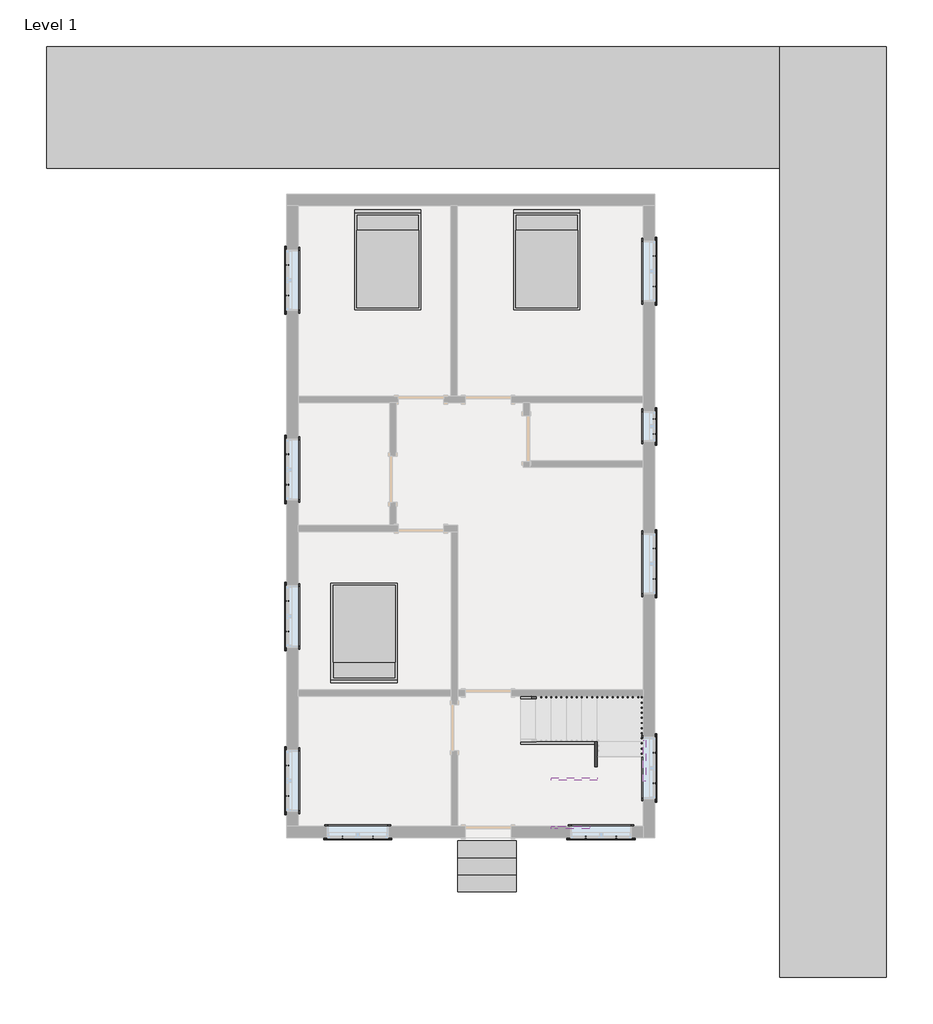
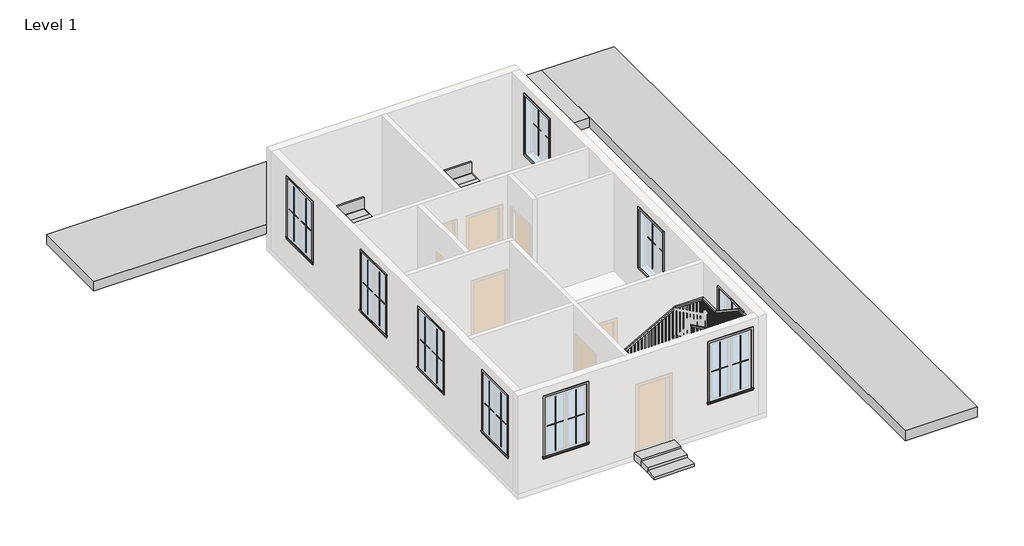
# One storey, part 2 of 2: 43 proxies, 6 members, 3 furniture elements, 1 railing.
"""IFC4 building model written with IfcOpenShell, lengths in millimetres."""

from ifc_helpers import new_model, si_unit, frame, origin, place, context, project, spatial, polyline, outline, extrude, faceted_brep, transform, mapped, element, save
from components import generic_models_1_generic_models_1_13bb2270, generic_models_2_generic_models_2_8d9d6b08, generic_models_3_generic_models_3_c7f04afc, muntin_pattern_2x2_muntin_pattern_2x2_2b4d9f72, muntin_pattern_2x2_muntin_pattern_2x2_ef995ed3, muntin_pattern_2x2_muntin_pattern_2x2_53152e2c, muntin_pattern_2x2_muntin_pattern_2x2_e8f3e573, trim_window_exterior_flat_with_sill_b7e4d11c, trim_window_exterior_flat_with_sill_a665a915, trim_window_interior_flat_picture_frame_936b8d2a, trim_window_interior_flat_picture_frame_d485c387, bed_17739_bed_17739_15c61121

model = new_model("IFC4")

# Units and contexts
model_context = context("Model", 3, world=origin())
ifc_project = project(units=[si_unit("LENGTHUNIT", "METRE", prefix="MILLI")], contexts=[model_context])

# Site, building, storey
site = spatial("IfcSite", under=ifc_project)
building = spatial("IfcBuilding", under=site)
storey = spatial("IfcBuildingStorey", under=building, Name="Level 1", Elevation=0.0)

# Proxies
placement = place(None, origin())
generic_models_1_generic_models_1_shape = generic_models_1_generic_models_1_13bb2270(model_context)
element("IfcBuildingElementProxy", 1, Name="Generic Models 1 : Generic Models 1", ObjectType="Generic Models 1 : Generic Models 1", at=placement, inside=storey, context=model_context, shape_type="MappedRepresentation", body=[
    mapped(generic_models_1_generic_models_1_shape, transform((0.0, 0.0, 0.0), x_axis=(1.0, 0.0, 0.0), y_axis=(0.0, 1.0, 0.0), z_axis=(0.0, 0.0, 1.0))),
])
generic_models_2_generic_models_2_shape = generic_models_2_generic_models_2_8d9d6b08(model_context)
element("IfcBuildingElementProxy", 2, Name="Generic Models 2 : Generic Models 2", ObjectType="Generic Models 2 : Generic Models 2", at=placement, inside=storey, context=model_context, shape_type="MappedRepresentation", body=[
    mapped(generic_models_2_generic_models_2_shape, transform((0.0, 0.0, 0.0), x_axis=(1.0, 0.0, 0.0), y_axis=(0.0, 1.0, 0.0), z_axis=(0.0, 0.0, 1.0))),
])
generic_models_3_generic_models_3_shape = generic_models_3_generic_models_3_c7f04afc(model_context)
element("IfcBuildingElementProxy", 3, Name="Generic Models 3 : Generic Models 3", ObjectType="Generic Models 3 : Generic Models 3", at=placement, inside=storey, context=model_context, shape_type="MappedRepresentation", body=[
    mapped(generic_models_3_generic_models_3_shape, transform((0.0, 0.0, 0.0), x_axis=(1.0, 0.0, 0.0), y_axis=(0.0, 1.0, 0.0), z_axis=(0.0, 0.0, 1.0))),
])
muntin_pattern_2x2_muntin_pattern_2x2_shape = muntin_pattern_2x2_muntin_pattern_2x2_2b4d9f72(model_context)
element("IfcBuildingElementProxy", 4, Name="Muntin Pattern_2x2 : Muntin Pattern_2x2", ObjectType="Muntin Pattern_2x2 : Muntin Pattern_2x2", at=placement, inside=storey, context=model_context, shape_type="MappedRepresentation", body=[
    mapped(muntin_pattern_2x2_muntin_pattern_2x2_shape, transform((1025.525, 12434.8875, 984.25), x_axis=(0.0, 1.0, 0.0), y_axis=(-1.0, 0.0, 0.0), z_axis=(0.0, 0.0, 1.0))),
])
element("IfcBuildingElementProxy", 5, Name="Muntin Pattern_2x2 : Muntin Pattern_2x2", ObjectType="Muntin Pattern_2x2 : Muntin Pattern_2x2", at=placement, inside=storey, context=model_context, shape_type="MappedRepresentation", body=[
    mapped(muntin_pattern_2x2_muntin_pattern_2x2_shape, transform((8321.675, 13219.1125, 984.25), x_axis=(0.0, -1.0, 0.0), y_axis=(1.0, 0.0, 0.0), z_axis=(0.0, 0.0, 1.0))),
])
element("IfcBuildingElementProxy", 6, Name="Muntin Pattern_2x2 : Muntin Pattern_2x2", ObjectType="Muntin Pattern_2x2 : Muntin Pattern_2x2", at=placement, inside=storey, context=model_context, shape_type="MappedRepresentation", body=[
    mapped(muntin_pattern_2x2_muntin_pattern_2x2_shape, transform((8321.675, 3338.5125, 984.25), x_axis=(0.0, -1.0, 0.0), y_axis=(1.0, 0.0, 0.0), z_axis=(0.0, 0.0, 1.0))),
])
element("IfcBuildingElementProxy", 7, Name="Muntin Pattern_2x2 : Muntin Pattern_2x2", ObjectType="Muntin Pattern_2x2 : Muntin Pattern_2x2", at=placement, inside=storey, context=model_context, shape_type="MappedRepresentation", body=[
    mapped(muntin_pattern_2x2_muntin_pattern_2x2_shape, transform((7567.6125, 1660.525, 984.25), x_axis=(-1.0, 0.0, 0.0), y_axis=(0.0, -1.0, 0.0), z_axis=(0.0, 0.0, 1.0))),
])
element("IfcBuildingElementProxy", 8, Name="Muntin Pattern_2x2 : Muntin Pattern_2x2", ObjectType="Muntin Pattern_2x2 : Muntin Pattern_2x2", at=placement, inside=storey, context=model_context, shape_type="MappedRepresentation", body=[
    mapped(muntin_pattern_2x2_muntin_pattern_2x2_shape, transform((2728.9125, 1660.525, 984.25), x_axis=(-1.0, 0.0, 0.0), y_axis=(0.0, -1.0, 0.0), z_axis=(0.0, 0.0, 1.0))),
])
element("IfcBuildingElementProxy", 9, Name="Muntin Pattern_2x2 : Muntin Pattern_2x2", ObjectType="Muntin Pattern_2x2 : Muntin Pattern_2x2", at=placement, inside=storey, context=model_context, shape_type="MappedRepresentation", body=[
    mapped(muntin_pattern_2x2_muntin_pattern_2x2_shape, transform((1025.525, 2478.0875, 984.25), x_axis=(0.0, 1.0, 0.0), y_axis=(-1.0, 0.0, 0.0), z_axis=(0.0, 0.0, 1.0))),
])
element("IfcBuildingElementProxy", 10, Name="Muntin Pattern_2x2 : Muntin Pattern_2x2", ObjectType="Muntin Pattern_2x2 : Muntin Pattern_2x2", at=placement, inside=storey, context=model_context, shape_type="MappedRepresentation", body=[
    mapped(muntin_pattern_2x2_muntin_pattern_2x2_shape, transform((1025.525, 5748.3375, 984.25), x_axis=(0.0, 1.0, 0.0), y_axis=(-1.0, 0.0, 0.0), z_axis=(0.0, 0.0, 1.0))),
])
element("IfcBuildingElementProxy", 11, Name="Muntin Pattern_2x2 : Muntin Pattern_2x2", ObjectType="Muntin Pattern_2x2 : Muntin Pattern_2x2", at=placement, inside=storey, context=model_context, shape_type="MappedRepresentation", body=[
    mapped(muntin_pattern_2x2_muntin_pattern_2x2_shape, transform((1025.525, 8669.3375, 984.25), x_axis=(0.0, 1.0, 0.0), y_axis=(-1.0, 0.0, 0.0), z_axis=(0.0, 0.0, 1.0))),
])
element("IfcBuildingElementProxy", 12, Name="Muntin Pattern_2x2 : Muntin Pattern_2x2", ObjectType="Muntin Pattern_2x2 : Muntin Pattern_2x2", at=placement, inside=storey, context=model_context, shape_type="MappedRepresentation", body=[
    mapped(muntin_pattern_2x2_muntin_pattern_2x2_shape, transform((8321.675, 7402.5125, 984.25), x_axis=(0.0, -1.0, 0.0), y_axis=(1.0, 0.0, 0.0), z_axis=(0.0, 0.0, 1.0))),
])
muntin_pattern_2x2_muntin_pattern_2x2_2_shape = muntin_pattern_2x2_muntin_pattern_2x2_ef995ed3(model_context)
element("IfcBuildingElementProxy", 13, Name="Muntin Pattern_2x2 : Muntin Pattern_2x2", ObjectType="Muntin Pattern_2x2 : Muntin Pattern_2x2", at=placement, inside=storey, context=model_context, shape_type="MappedRepresentation", body=[
    mapped(muntin_pattern_2x2_muntin_pattern_2x2_2_shape, transform((1025.525, 13041.3125, 984.25), x_axis=(0.0, -1.0, 0.0), y_axis=(1.0, 0.0, 0.0), z_axis=(0.0, 0.0, 1.0))),
])
element("IfcBuildingElementProxy", 14, Name="Muntin Pattern_2x2 : Muntin Pattern_2x2", ObjectType="Muntin Pattern_2x2 : Muntin Pattern_2x2", at=placement, inside=storey, context=model_context, shape_type="MappedRepresentation", body=[
    mapped(muntin_pattern_2x2_muntin_pattern_2x2_2_shape, transform((8321.675, 12612.6875, 984.25), x_axis=(0.0, 1.0, 0.0), y_axis=(-1.0, 0.0, 0.0), z_axis=(0.0, 0.0, 1.0))),
])
element("IfcBuildingElementProxy", 15, Name="Muntin Pattern_2x2 : Muntin Pattern_2x2", ObjectType="Muntin Pattern_2x2 : Muntin Pattern_2x2", at=placement, inside=storey, context=model_context, shape_type="MappedRepresentation", body=[
    mapped(muntin_pattern_2x2_muntin_pattern_2x2_2_shape, transform((8321.675, 2732.0875, 984.25), x_axis=(0.0, 1.0, 0.0), y_axis=(-1.0, 0.0, 0.0), z_axis=(0.0, 0.0, 1.0))),
])
element("IfcBuildingElementProxy", 16, Name="Muntin Pattern_2x2 : Muntin Pattern_2x2", ObjectType="Muntin Pattern_2x2 : Muntin Pattern_2x2", at=placement, inside=storey, context=model_context, shape_type="MappedRepresentation", body=[
    mapped(muntin_pattern_2x2_muntin_pattern_2x2_2_shape, transform((6961.1875, 1660.525, 984.25), x_axis=(1.0, 0.0, 0.0), y_axis=(0.0, 1.0, 0.0), z_axis=(0.0, 0.0, 1.0))),
])
element("IfcBuildingElementProxy", 17, Name="Muntin Pattern_2x2 : Muntin Pattern_2x2", ObjectType="Muntin Pattern_2x2 : Muntin Pattern_2x2", at=placement, inside=storey, context=model_context, shape_type="MappedRepresentation", body=[
    mapped(muntin_pattern_2x2_muntin_pattern_2x2_2_shape, transform((2122.4875, 1660.525, 984.25), x_axis=(1.0, 0.0, 0.0), y_axis=(0.0, 1.0, 0.0), z_axis=(0.0, 0.0, 1.0))),
])
element("IfcBuildingElementProxy", 18, Name="Muntin Pattern_2x2 : Muntin Pattern_2x2", ObjectType="Muntin Pattern_2x2 : Muntin Pattern_2x2", at=placement, inside=storey, context=model_context, shape_type="MappedRepresentation", body=[
    mapped(muntin_pattern_2x2_muntin_pattern_2x2_2_shape, transform((1025.525, 3084.5125, 984.25), x_axis=(0.0, -1.0, 0.0), y_axis=(1.0, 0.0, 0.0), z_axis=(0.0, 0.0, 1.0))),
])
element("IfcBuildingElementProxy", 19, Name="Muntin Pattern_2x2 : Muntin Pattern_2x2", ObjectType="Muntin Pattern_2x2 : Muntin Pattern_2x2", at=placement, inside=storey, context=model_context, shape_type="MappedRepresentation", body=[
    mapped(muntin_pattern_2x2_muntin_pattern_2x2_2_shape, transform((1025.525, 6354.7625, 984.25), x_axis=(0.0, -1.0, 0.0), y_axis=(1.0, 0.0, 0.0), z_axis=(0.0, 0.0, 1.0))),
])
element("IfcBuildingElementProxy", 20, Name="Muntin Pattern_2x2 : Muntin Pattern_2x2", ObjectType="Muntin Pattern_2x2 : Muntin Pattern_2x2", at=placement, inside=storey, context=model_context, shape_type="MappedRepresentation", body=[
    mapped(muntin_pattern_2x2_muntin_pattern_2x2_2_shape, transform((1025.525, 9275.7625, 984.25), x_axis=(0.0, -1.0, 0.0), y_axis=(1.0, 0.0, 0.0), z_axis=(0.0, 0.0, 1.0))),
])
element("IfcBuildingElementProxy", 21, Name="Muntin Pattern_2x2 : Muntin Pattern_2x2", ObjectType="Muntin Pattern_2x2 : Muntin Pattern_2x2", at=placement, inside=storey, context=model_context, shape_type="MappedRepresentation", body=[
    mapped(muntin_pattern_2x2_muntin_pattern_2x2_2_shape, transform((8321.675, 6796.0875, 984.25), x_axis=(0.0, 1.0, 0.0), y_axis=(-1.0, 0.0, 0.0), z_axis=(0.0, 0.0, 1.0))),
])
muntin_pattern_2x2_muntin_pattern_2x2_3_shape = muntin_pattern_2x2_muntin_pattern_2x2_53152e2c(model_context)
element("IfcBuildingElementProxy", 22, Name="Muntin Pattern_2x2 : Muntin Pattern_2x2", ObjectType="Muntin Pattern_2x2 : Muntin Pattern_2x2", at=placement, inside=storey, context=model_context, shape_type="MappedRepresentation", body=[
    mapped(muntin_pattern_2x2_muntin_pattern_2x2_3_shape, transform((8321.675, 9980.6125, 984.25), x_axis=(0.0, -1.0, 0.0), y_axis=(1.0, 0.0, 0.0), z_axis=(0.0, 0.0, 1.0))),
])
muntin_pattern_2x2_muntin_pattern_2x2_4_shape = muntin_pattern_2x2_muntin_pattern_2x2_e8f3e573(model_context)
element("IfcBuildingElementProxy", 23, Name="Muntin Pattern_2x2 : Muntin Pattern_2x2", ObjectType="Muntin Pattern_2x2 : Muntin Pattern_2x2", at=placement, inside=storey, context=model_context, shape_type="MappedRepresentation", body=[
    mapped(muntin_pattern_2x2_muntin_pattern_2x2_4_shape, transform((8321.675, 9678.9875, 984.25), x_axis=(0.0, 1.0, 0.0), y_axis=(-1.0, 0.0, 0.0), z_axis=(0.0, 0.0, 1.0))),
])
trim_window_exterior_flat_with_sill_shape = trim_window_exterior_flat_with_sill_b7e4d11c(model_context)
element("IfcBuildingElementProxy", 24, Name="Trim-Window-Exterior-Flat : with Sill", ObjectType="Trim-Window-Exterior-Flat : with Sill", at=placement, inside=storey, context=model_context, shape_type="MappedRepresentation", body=[
    mapped(trim_window_exterior_flat_with_sill_shape, transform((1016.0, 12738.1, 2743.2), x_axis=(0.0, -1.0, 0.0), y_axis=(0.0, 0.0, 1.0), z_axis=(-1.0, 0.0, 0.0))),
])
element("IfcBuildingElementProxy", 25, Name="Trim-Window-Exterior-Flat : with Sill", ObjectType="Trim-Window-Exterior-Flat : with Sill", at=placement, inside=storey, context=model_context, shape_type="MappedRepresentation", body=[
    mapped(trim_window_exterior_flat_with_sill_shape, transform((8331.2, 12915.9, 2743.2), x_axis=(0.0, 1.0, 0.0), y_axis=(0.0, 0.0, 1.0), z_axis=(1.0, 0.0, 0.0))),
])
element("IfcBuildingElementProxy", 26, Name="Trim-Window-Exterior-Flat : with Sill", ObjectType="Trim-Window-Exterior-Flat : with Sill", at=placement, inside=storey, context=model_context, shape_type="MappedRepresentation", body=[
    mapped(trim_window_exterior_flat_with_sill_shape, transform((8331.2, 3035.3, 2743.2), x_axis=(0.0, 1.0, 0.0), y_axis=(0.0, 0.0, 1.0), z_axis=(1.0, 0.0, 0.0))),
])
element("IfcBuildingElementProxy", 27, Name="Trim-Window-Exterior-Flat : with Sill", ObjectType="Trim-Window-Exterior-Flat : with Sill", at=placement, inside=storey, context=model_context, shape_type="MappedRepresentation", body=[
    mapped(trim_window_exterior_flat_with_sill_shape, transform((7264.4, 1651.0, 2743.2), x_axis=(1.0, 0.0, 0.0), y_axis=(0.0, 0.0, 1.0), z_axis=(0.0, -1.0, 0.0))),
])
element("IfcBuildingElementProxy", 28, Name="Trim-Window-Exterior-Flat : with Sill", ObjectType="Trim-Window-Exterior-Flat : with Sill", at=placement, inside=storey, context=model_context, shape_type="MappedRepresentation", body=[
    mapped(trim_window_exterior_flat_with_sill_shape, transform((2425.7, 1651.0, 2743.2), x_axis=(1.0, 0.0, 0.0), y_axis=(0.0, 0.0, 1.0), z_axis=(0.0, -1.0, 0.0))),
])
element("IfcBuildingElementProxy", 29, Name="Trim-Window-Exterior-Flat : with Sill", ObjectType="Trim-Window-Exterior-Flat : with Sill", at=placement, inside=storey, context=model_context, shape_type="MappedRepresentation", body=[
    mapped(trim_window_exterior_flat_with_sill_shape, transform((1016.0, 2781.3, 2743.2), x_axis=(0.0, -1.0, 0.0), y_axis=(0.0, 0.0, 1.0), z_axis=(-1.0, 0.0, 0.0))),
])
element("IfcBuildingElementProxy", 30, Name="Trim-Window-Exterior-Flat : with Sill", ObjectType="Trim-Window-Exterior-Flat : with Sill", at=placement, inside=storey, context=model_context, shape_type="MappedRepresentation", body=[
    mapped(trim_window_exterior_flat_with_sill_shape, transform((1016.0, 6051.55, 2743.2), x_axis=(0.0, -1.0, 0.0), y_axis=(0.0, 0.0, 1.0), z_axis=(-1.0, 0.0, 0.0))),
])
element("IfcBuildingElementProxy", 31, Name="Trim-Window-Exterior-Flat : with Sill", ObjectType="Trim-Window-Exterior-Flat : with Sill", at=placement, inside=storey, context=model_context, shape_type="MappedRepresentation", body=[
    mapped(trim_window_exterior_flat_with_sill_shape, transform((1016.0, 8972.55, 2743.2), x_axis=(0.0, -1.0, 0.0), y_axis=(0.0, 0.0, 1.0), z_axis=(-1.0, 0.0, 0.0))),
])
element("IfcBuildingElementProxy", 32, Name="Trim-Window-Exterior-Flat : with Sill", ObjectType="Trim-Window-Exterior-Flat : with Sill", at=placement, inside=storey, context=model_context, shape_type="MappedRepresentation", body=[
    mapped(trim_window_exterior_flat_with_sill_shape, transform((8331.2, 7099.3, 2743.2), x_axis=(0.0, 1.0, 0.0), y_axis=(0.0, 0.0, 1.0), z_axis=(1.0, 0.0, 0.0))),
])
trim_window_exterior_flat_with_sill_2_shape = trim_window_exterior_flat_with_sill_a665a915(model_context)
element("IfcBuildingElementProxy", 33, Name="Trim-Window-Exterior-Flat : with Sill", ObjectType="Trim-Window-Exterior-Flat : with Sill", at=placement, inside=storey, context=model_context, shape_type="MappedRepresentation", body=[
    mapped(trim_window_exterior_flat_with_sill_2_shape, transform((8331.2, 9829.8, 1828.8), x_axis=(0.0, 1.0, 0.0), y_axis=(0.0, 0.0, 1.0), z_axis=(1.0, 0.0, 0.0))),
])
trim_window_interior_flat_picture_frame_shape = trim_window_interior_flat_picture_frame_936b8d2a(model_context)
element("IfcBuildingElementProxy", 34, Name="Trim-Window-Interior-Flat : Picture Frame", ObjectType="Trim-Window-Interior-Flat : Picture Frame", at=placement, inside=storey, context=model_context, shape_type="MappedRepresentation", body=[
    mapped(trim_window_interior_flat_picture_frame_shape, transform((1244.6, 12738.1, 2743.2), x_axis=(0.0, 1.0, 0.0), y_axis=(0.0, 0.0, 1.0), z_axis=(1.0, 0.0, 0.0))),
])
element("IfcBuildingElementProxy", 35, Name="Trim-Window-Interior-Flat : Picture Frame", ObjectType="Trim-Window-Interior-Flat : Picture Frame", at=placement, inside=storey, context=model_context, shape_type="MappedRepresentation", body=[
    mapped(trim_window_interior_flat_picture_frame_shape, transform((8102.6, 12915.9, 2743.2), x_axis=(0.0, -1.0, 0.0), y_axis=(0.0, 0.0, 1.0), z_axis=(-1.0, 0.0, 0.0))),
])
element("IfcBuildingElementProxy", 36, Name="Trim-Window-Interior-Flat : Picture Frame", ObjectType="Trim-Window-Interior-Flat : Picture Frame", at=placement, inside=storey, context=model_context, shape_type="MappedRepresentation", body=[
    mapped(trim_window_interior_flat_picture_frame_shape, transform((8102.6, 3035.3, 2743.2), x_axis=(0.0, -1.0, 0.0), y_axis=(0.0, 0.0, 1.0), z_axis=(-1.0, 0.0, 0.0))),
])
element("IfcBuildingElementProxy", 37, Name="Trim-Window-Interior-Flat : Picture Frame", ObjectType="Trim-Window-Interior-Flat : Picture Frame", at=placement, inside=storey, context=model_context, shape_type="MappedRepresentation", body=[
    mapped(trim_window_interior_flat_picture_frame_shape, transform((7264.4, 1879.6, 2743.2), x_axis=(-1.0, 0.0, 0.0), y_axis=(0.0, 0.0, 1.0), z_axis=(0.0, 1.0, 0.0))),
])
element("IfcBuildingElementProxy", 38, Name="Trim-Window-Interior-Flat : Picture Frame", ObjectType="Trim-Window-Interior-Flat : Picture Frame", at=placement, inside=storey, context=model_context, shape_type="MappedRepresentation", body=[
    mapped(trim_window_interior_flat_picture_frame_shape, transform((2425.7, 1879.6, 2743.2), x_axis=(-1.0, 0.0, 0.0), y_axis=(0.0, 0.0, 1.0), z_axis=(0.0, 1.0, 0.0))),
])
element("IfcBuildingElementProxy", 39, Name="Trim-Window-Interior-Flat : Picture Frame", ObjectType="Trim-Window-Interior-Flat : Picture Frame", at=placement, inside=storey, context=model_context, shape_type="MappedRepresentation", body=[
    mapped(trim_window_interior_flat_picture_frame_shape, transform((1244.6, 2781.3, 2743.2), x_axis=(0.0, 1.0, 0.0), y_axis=(0.0, 0.0, 1.0), z_axis=(1.0, 0.0, 0.0))),
])
element("IfcBuildingElementProxy", 40, Name="Trim-Window-Interior-Flat : Picture Frame", ObjectType="Trim-Window-Interior-Flat : Picture Frame", at=placement, inside=storey, context=model_context, shape_type="MappedRepresentation", body=[
    mapped(trim_window_interior_flat_picture_frame_shape, transform((1244.6, 6051.55, 2743.2), x_axis=(0.0, 1.0, 0.0), y_axis=(0.0, 0.0, 1.0), z_axis=(1.0, 0.0, 0.0))),
])
element("IfcBuildingElementProxy", 41, Name="Trim-Window-Interior-Flat : Picture Frame", ObjectType="Trim-Window-Interior-Flat : Picture Frame", at=placement, inside=storey, context=model_context, shape_type="MappedRepresentation", body=[
    mapped(trim_window_interior_flat_picture_frame_shape, transform((1244.6, 8972.55, 2743.2), x_axis=(0.0, 1.0, 0.0), y_axis=(0.0, 0.0, 1.0), z_axis=(1.0, 0.0, 0.0))),
])
element("IfcBuildingElementProxy", 42, Name="Trim-Window-Interior-Flat : Picture Frame", ObjectType="Trim-Window-Interior-Flat : Picture Frame", at=placement, inside=storey, context=model_context, shape_type="MappedRepresentation", body=[
    mapped(trim_window_interior_flat_picture_frame_shape, transform((8102.6, 7099.3, 2743.2), x_axis=(0.0, -1.0, 0.0), y_axis=(0.0, 0.0, 1.0), z_axis=(-1.0, 0.0, 0.0))),
])
trim_window_interior_flat_picture_frame_2_shape = trim_window_interior_flat_picture_frame_d485c387(model_context)
element("IfcBuildingElementProxy", 43, Name="Trim-Window-Interior-Flat : Picture Frame", ObjectType="Trim-Window-Interior-Flat : Picture Frame", at=placement, inside=storey, context=model_context, shape_type="MappedRepresentation", body=[
    mapped(trim_window_interior_flat_picture_frame_2_shape, transform((8102.6, 9829.8, 1828.8), x_axis=(0.0, -1.0, 0.0), y_axis=(0.0, 0.0, 1.0), z_axis=(-1.0, 0.0, 0.0))),
])

# Furniture
bed_17739_bed_17739_shape = bed_17739_bed_17739_15c61121(model_context)
element("IfcFurniture", 44, ObjectType="Bed_17739 : Bed_17739", at=placement, inside=storey, context=model_context, shape_type="MappedRepresentation", body=[
    mapped(bed_17739_bed_17739_shape, transform((3022.6, 13119.1, 0.0), x_axis=(1.0, 0.0, 0.0), y_axis=(0.0, 1.0, 0.0), z_axis=(0.0, 0.0, 1.0))),
])
element("IfcFurniture", 45, ObjectType="Bed_17739 : Bed_17739", at=placement, inside=storey, context=model_context, shape_type="MappedRepresentation", body=[
    mapped(bed_17739_bed_17739_shape, transform((6184.9, 13119.1, 0.0), x_axis=(1.0, 0.0, 0.0), y_axis=(0.0, 1.0, 0.0), z_axis=(0.0, 0.0, 1.0))),
])
element("IfcFurniture", 46, ObjectType="Bed_17739 : Bed_17739", at=placement, inside=storey, context=model_context, shape_type="MappedRepresentation", body=[
    mapped(bed_17739_bed_17739_shape, transform((2552.7, 5746.75, 0.0), x_axis=(-1.0, 0.0, 0.0), y_axis=(0.0, -1.0, 0.0), z_axis=(0.0, 0.0, 1.0))),
])

# Members
element("IfcMember", 47, ObjectType="Stringer - 2\" Width", at=placement, inside=storey, context=model_context, shape_type="SweptSolid", body=[
    extrude(outline(polyline([(207.5983948, 5664.2), (0.0, 5664.2), (0.0, 5918.1445028), (628.6731743, 7049.7562165), (628.6731743, 6422.1346031), (207.5983948, 5664.2)])), frame((0.0, 4464.05, 0.0), z_axis=(0.0, 1.0, 0.0), x_axis=(0.0, 0.0, 1.0)), (0.0, 0.0, 1.0), 50.8),
])
element("IfcMember", 48, ObjectType="Stringer - 2\" Width", at=placement, inside=storey, context=model_context, shape_type="SweptSolid", body=[
    extrude(outline(polyline([(3037.194166, 1213.5863873), (2767.4296295, 1393.4294117), (3316.9156438, 1393.4294117), (3586.6801804, 1213.5863873), (3037.194166, 1213.5863873)])), frame((8102.6, 0.0, 0.0), z_axis=(1.0, 0.0, 0.0), x_axis=(0.0, 1.0, 0.0)), (0.0, 0.0, 1.0), 50.8),
])
element("IfcMember", 49, ObjectType="Stringer - 2\" Width", at=placement, inside=storey, context=model_context, shape_type="SweptSolid", body=[
    extrude(outline(polyline([(1985.3158313, 7036.0519338), (2408.6974859, 6273.1405542), (2060.1076387, 6273.1405542), (1985.3158313, 6407.9114408), (1985.3158313, 7036.0519338)])), frame((0.0, 1828.8, 0.0), z_axis=(0.0, 1.0, 0.0), x_axis=(0.0, 0.0, 1.0)), (0.0, 0.0, 1.0), 50.8),
])
element("IfcMember", 50, ObjectType="Stringer - 2\" Width", at=placement, inside=storey, context=model_context, shape_type="SweptSolid", body=[
    extrude(outline(polyline([(207.5983948, 5664.2), (0.0, 5664.2), (0.0, 5918.1445028), (677.3641651, 7137.4), (1026.0428392, 7137.4), (207.5983948, 5664.2)])), frame((0.0, 3505.2, 0.0), z_axis=(0.0, 1.0, 0.0), x_axis=(0.0, 0.0, 1.0)), (0.0, 0.0, 1.0), 50.8),
])
element("IfcMember", 51, ObjectType="Stringer - 2\" Width", at=placement, inside=storey, context=model_context, shape_type="SweptSolid", body=[
    extrude(outline(polyline([(3556.0, 1234.0398409), (3556.0, 867.7158313), (2844.8, 1341.8491647), (2844.8, 1708.1731743), (3556.0, 1234.0398409)])), frame((7137.4, 0.0, 0.0), z_axis=(1.0, 0.0, 0.0), x_axis=(0.0, 1.0, 0.0)), (0.0, 0.0, 1.0), 50.8),
])
element("IfcMember", 52, ObjectType="Stringer - 2\" Width", at=placement, inside=storey, context=model_context, shape_type="SweptSolid", body=[
    extrude(outline(polyline([(1552.2906202, 7188.2), (1900.8804673, 7188.2), (2408.6974859, 6273.1405542), (2060.1076387, 6273.1405542), (1552.2906202, 7188.2)])), frame((0.0, 2794.0, 0.0), z_axis=(0.0, 1.0, 0.0), x_axis=(0.0, 0.0, 1.0)), (0.0, 0.0, 1.0), 50.8),
])

# Railing
element("IfcRailing", 53, ObjectType="Handrail - Rectangular", at=placement, inside=storey, context=model_context, shape_type="SolidModel", body=[
    faceted_brep([(5664.2, 4464.05, 1083.7333333), (5664.2, 4464.05, 1025.620221), (5664.2, 4413.25, 1025.620221), (5664.2, 4413.25, 1083.7333333), (7255.51, 4464.05, 1967.7944444), (7268.6736022, 4464.05, 1916.9944444), (7268.6736022, 4413.25, 1916.9944444), (7255.51, 4413.25, 1967.7944444), (8102.6, 4464.05, 1967.7944444), (8102.6, 4464.05, 1916.9944444), (8051.8, 4413.25, 1916.9944444), (8051.8, 4413.25, 1967.7944444), (8102.6, 3753.9083333, 1967.7944444), (8102.6, 3738.5273309, 1916.9944444), (8051.8, 3738.5273309, 1916.9944444), (8051.8, 3753.9083333, 1967.7944444), (8102.6, 2592.6497226, 2741.9668516), (8102.6, 2577.2687202, 2691.1668516), (8051.8, 2577.2687202, 2691.1668516), (8051.8, 2592.6497226, 2741.9668516), (8102.6, 1879.6, 2741.9668516), (8102.6, 1879.6, 2691.1668516), (8051.8, 1930.4, 2691.1668516), (8051.8, 1930.4, 2741.9668516), (7251.4252309, 1879.6, 2741.9668516), (7238.2699224, 1879.6, 2691.1668516), (7238.2699224, 1930.4, 2691.1668516), (7251.4252309, 1930.4, 2741.9668516), (6273.1405542, 1879.6, 3285.0666667), (6273.1405542, 1930.4, 3285.0666667), (6273.1405542, 1930.4, 3226.9634289), (6273.1405542, 1879.6, 3226.9634289)], [[[0, 1, 2, 3]], [[1, 0, 4, 5]], [[2, 1, 5, 6]], [[3, 2, 6, 7]], [[0, 3, 7, 4]], [[5, 4, 8, 9]], [[6, 5, 9, 10]], [[7, 6, 10, 11]], [[4, 7, 11, 8]], [[9, 8, 12, 13]], [[10, 9, 13, 14]], [[11, 10, 14, 15]], [[8, 11, 15, 12]], [[13, 12, 16, 17]], [[14, 13, 17, 18]], [[15, 14, 18, 19]], [[12, 15, 19, 16]], [[17, 16, 20, 21]], [[18, 17, 21, 22]], [[19, 18, 22, 23]], [[16, 19, 23, 20]], [[21, 20, 24, 25]], [[22, 21, 25, 26]], [[23, 22, 26, 27]], [[20, 23, 27, 24]], [[28, 29, 30, 31]], [[25, 24, 28, 31]], [[26, 25, 31, 30]], [[27, 26, 30, 29]], [[24, 27, 29, 28]]]),
    extrude(outline(polyline([(3189.5823619, 6340.475), (2201.3333333, 6340.475), (2201.3333333, 6359.525), (3179.0066555, 6359.525), (3189.5823619, 6340.475)])), frame((0.0, 1895.475, 0.0), z_axis=(0.0, 1.0, 0.0), x_axis=(0.0, 0.0, 1.0)), (0.0, 0.0, 1.0), 19.05),
    extrude(outline(polyline([(3133.1785946, 6442.075), (2201.3333333, 6442.075), (2201.3333333, 6461.125), (3122.6028883, 6461.125), (3133.1785946, 6442.075)])), frame((0.0, 1895.475, 0.0), z_axis=(0.0, 1.0, 0.0), x_axis=(0.0, 0.0, 1.0)), (0.0, 0.0, 1.0), 19.05),
    extrude(outline(polyline([(3076.7748274, 6543.675), (2201.3333333, 6543.675), (2201.3333333, 6562.725), (3066.199121, 6562.725), (3076.7748274, 6543.675)])), frame((0.0, 1895.475, 0.0), z_axis=(0.0, 1.0, 0.0), x_axis=(0.0, 0.0, 1.0)), (0.0, 0.0, 1.0), 19.05),
    extrude(outline(polyline([(3020.2490285, 6645.275), (2032.0, 6645.275), (2032.0, 6664.325), (3009.6733222, 6664.325), (3020.2490285, 6645.275)])), frame((0.0, 1895.475, 0.0), z_axis=(0.0, 1.0, 0.0), x_axis=(0.0, 0.0, 1.0)), (0.0, 0.0, 1.0), 19.05),
    extrude(outline(polyline([(2963.8452613, 6746.875), (2032.0, 6746.875), (2032.0, 6765.925), (2953.2695549, 6765.925), (2963.8452613, 6746.875)])), frame((0.0, 1895.475, 0.0), z_axis=(0.0, 1.0, 0.0), x_axis=(0.0, 0.0, 1.0)), (0.0, 0.0, 1.0), 19.05),
    extrude(outline(polyline([(2907.441494, 6848.475), (2032.0, 6848.475), (2032.0, 6867.525), (2896.8657877, 6867.525), (2907.441494, 6848.475)])), frame((0.0, 1895.475, 0.0), z_axis=(0.0, 1.0, 0.0), x_axis=(0.0, 0.0, 1.0)), (0.0, 0.0, 1.0), 19.05),
    extrude(outline(polyline([(2851.1597584, 6950.075), (1862.6666667, 6950.075), (1862.6666667, 6969.125), (2840.584052, 6969.125), (2851.1597584, 6950.075)])), frame((0.0, 1895.475, 0.0), z_axis=(0.0, 1.0, 0.0), x_axis=(0.0, 0.0, 1.0)), (0.0, 0.0, 1.0), 19.05),
    extrude(outline(polyline([(2794.7559911, 7051.675), (1862.6666667, 7051.675), (1862.6666667, 7070.725), (2784.1802848, 7070.725), (2794.7559911, 7051.675)])), frame((0.0, 1895.475, 0.0), z_axis=(0.0, 1.0, 0.0), x_axis=(0.0, 0.0, 1.0)), (0.0, 0.0, 1.0), 19.05),
    extrude(outline(polyline([(2738.3522239, 7153.275), (1862.6666667, 7153.275), (1862.6666667, 7172.325), (2727.7765175, 7172.325), (2738.3522239, 7153.275)])), frame((0.0, 1895.475, 0.0), z_axis=(0.0, 1.0, 0.0), x_axis=(0.0, 0.0, 1.0)), (0.0, 0.0, 1.0), 19.05),
    extrude(outline(polyline([(7273.925, 1895.475), (7254.875, 1895.475), (7254.875, 1914.525), (7273.925, 1914.525), (7273.925, 1895.475)])), frame((0.0, 0.0, 1693.3333333), z_axis=(0.0, 0.0, 1.0), x_axis=(1.0, 0.0, 0.0)), (0.0, 0.0, 1.0), 997.8335183),
    extrude(outline(polyline([(7375.525, 1895.475), (7356.475, 1895.475), (7356.475, 1914.525), (7375.525, 1914.525), (7375.525, 1895.475)])), frame((0.0, 0.0, 1693.3333333), z_axis=(0.0, 0.0, 1.0), x_axis=(1.0, 0.0, 0.0)), (0.0, 0.0, 1.0), 997.8335183),
    extrude(outline(polyline([(7477.125, 1895.475), (7458.075, 1895.475), (7458.075, 1914.525), (7477.125, 1914.525), (7477.125, 1895.475)])), frame((0.0, 0.0, 1693.3333333), z_axis=(0.0, 0.0, 1.0), x_axis=(1.0, 0.0, 0.0)), (0.0, 0.0, 1.0), 997.8335183),
    extrude(outline(polyline([(7578.725, 1895.475), (7559.675, 1895.475), (7559.675, 1914.525), (7578.725, 1914.525), (7578.725, 1895.475)])), frame((0.0, 0.0, 1693.3333333), z_axis=(0.0, 0.0, 1.0), x_axis=(1.0, 0.0, 0.0)), (0.0, 0.0, 1.0), 997.8335183),
    extrude(outline(polyline([(7680.325, 1895.475), (7661.275, 1895.475), (7661.275, 1914.525), (7680.325, 1914.525), (7680.325, 1895.475)])), frame((0.0, 0.0, 1693.3333333), z_axis=(0.0, 0.0, 1.0), x_axis=(1.0, 0.0, 0.0)), (0.0, 0.0, 1.0), 997.8335183),
    extrude(outline(polyline([(7781.925, 1895.475), (7762.875, 1895.475), (7762.875, 1914.525), (7781.925, 1914.525), (7781.925, 1895.475)])), frame((0.0, 0.0, 1693.3333333), z_axis=(0.0, 0.0, 1.0), x_axis=(1.0, 0.0, 0.0)), (0.0, 0.0, 1.0), 997.8335183),
    extrude(outline(polyline([(7883.525, 1895.475), (7864.475, 1895.475), (7864.475, 1914.525), (7883.525, 1914.525), (7883.525, 1895.475)])), frame((0.0, 0.0, 1693.3333333), z_axis=(0.0, 0.0, 1.0), x_axis=(1.0, 0.0, 0.0)), (0.0, 0.0, 1.0), 997.8335183),
    extrude(outline(polyline([(7985.125, 1895.475), (7966.075, 1895.475), (7966.075, 1914.525), (7985.125, 1914.525), (7985.125, 1895.475)])), frame((0.0, 0.0, 1693.3333333), z_axis=(0.0, 0.0, 1.0), x_axis=(1.0, 0.0, 0.0)), (0.0, 0.0, 1.0), 997.8335183),
    extrude(outline(polyline([(8086.725, 2009.775), (8086.725, 1990.725), (8067.675, 1990.725), (8067.675, 2009.775), (8086.725, 2009.775)])), frame((0.0, 0.0, 1693.3333333), z_axis=(0.0, 0.0, 1.0), x_axis=(1.0, 0.0, 0.0)), (0.0, 0.0, 1.0), 997.8335183),
    extrude(outline(polyline([(8086.725, 2111.375), (8086.725, 2092.325), (8067.675, 2092.325), (8067.675, 2111.375), (8086.725, 2111.375)])), frame((0.0, 0.0, 1693.3333333), z_axis=(0.0, 0.0, 1.0), x_axis=(1.0, 0.0, 0.0)), (0.0, 0.0, 1.0), 997.8335183),
    extrude(outline(polyline([(8086.725, 2212.975), (8086.725, 2193.925), (8067.675, 2193.925), (8067.675, 2212.975), (8086.725, 2212.975)])), frame((0.0, 0.0, 1693.3333333), z_axis=(0.0, 0.0, 1.0), x_axis=(1.0, 0.0, 0.0)), (0.0, 0.0, 1.0), 997.8335183),
    extrude(outline(polyline([(8086.725, 2314.575), (8086.725, 2295.525), (8067.675, 2295.525), (8067.675, 2314.575), (8086.725, 2314.575)])), frame((0.0, 0.0, 1693.3333333), z_axis=(0.0, 0.0, 1.0), x_axis=(1.0, 0.0, 0.0)), (0.0, 0.0, 1.0), 997.8335183),
    extrude(outline(polyline([(8086.725, 2416.175), (8086.725, 2397.125), (8067.675, 2397.125), (8067.675, 2416.175), (8086.725, 2416.175)])), frame((0.0, 0.0, 1693.3333333), z_axis=(0.0, 0.0, 1.0), x_axis=(1.0, 0.0, 0.0)), (0.0, 0.0, 1.0), 997.8335183),
    extrude(outline(polyline([(8086.725, 2517.775), (8086.725, 2498.725), (8067.675, 2498.725), (8067.675, 2517.775), (8086.725, 2517.775)])), frame((0.0, 0.0, 1693.3333333), z_axis=(0.0, 0.0, 1.0), x_axis=(1.0, 0.0, 0.0)), (0.0, 0.0, 1.0), 997.8335183),
    extrude(outline(polyline([(2619.375, 2663.0959984), (2619.375, 1693.3333333), (2600.325, 1693.3333333), (2600.325, 2675.7959984), (2619.375, 2663.0959984)])), frame((8067.675, 0.0, 0.0), z_axis=(1.0, 0.0, 0.0), x_axis=(0.0, 1.0, 0.0)), (0.0, 0.0, 1.0), 19.05),
    extrude(outline(polyline([(2720.975, 2595.3626651), (2720.975, 1693.3333333), (2701.925, 1693.3333333), (2701.925, 2608.0626651), (2720.975, 2595.3626651)])), frame((8067.675, 0.0, 0.0), z_axis=(1.0, 0.0, 0.0), x_axis=(0.0, 1.0, 0.0)), (0.0, 0.0, 1.0), 19.05),
    extrude(outline(polyline([(2822.575, 2527.6293317), (2822.575, 1524.0), (2803.525, 1524.0), (2803.525, 2540.3293317), (2822.575, 2527.6293317)])), frame((8067.675, 0.0, 0.0), z_axis=(1.0, 0.0, 0.0), x_axis=(0.0, 1.0, 0.0)), (0.0, 0.0, 1.0), 19.05),
    extrude(outline(polyline([(2924.175, 2459.8959984), (2924.175, 1524.0), (2905.125, 1524.0), (2905.125, 2472.5959984), (2924.175, 2459.8959984)])), frame((8067.675, 0.0, 0.0), z_axis=(1.0, 0.0, 0.0), x_axis=(0.0, 1.0, 0.0)), (0.0, 0.0, 1.0), 19.05),
    extrude(outline(polyline([(3025.775, 2392.1626651), (3025.775, 1524.0), (3006.725, 1524.0), (3006.725, 2404.8626651), (3025.775, 2392.1626651)])), frame((8067.675, 0.0, 0.0), z_axis=(1.0, 0.0, 0.0), x_axis=(0.0, 1.0, 0.0)), (0.0, 0.0, 1.0), 19.05),
    extrude(outline(polyline([(3127.375, 2324.4293317), (3127.375, 1354.6666667), (3108.325, 1354.6666667), (3108.325, 2337.1293317), (3127.375, 2324.4293317)])), frame((8067.675, 0.0, 0.0), z_axis=(1.0, 0.0, 0.0), x_axis=(0.0, 1.0, 0.0)), (0.0, 0.0, 1.0), 19.05),
    extrude(outline(polyline([(3228.975, 2256.6959984), (3228.975, 1354.6666667), (3209.925, 1354.6666667), (3209.925, 2269.3959984), (3228.975, 2256.6959984)])), frame((8067.675, 0.0, 0.0), z_axis=(1.0, 0.0, 0.0), x_axis=(0.0, 1.0, 0.0)), (0.0, 0.0, 1.0), 19.05),
    extrude(outline(polyline([(3330.575, 2188.9626651), (3330.575, 1185.3333333), (3311.525, 1185.3333333), (3311.525, 2201.6626651), (3330.575, 2188.9626651)])), frame((8067.675, 0.0, 0.0), z_axis=(1.0, 0.0, 0.0), x_axis=(0.0, 1.0, 0.0)), (0.0, 0.0, 1.0), 19.05),
    extrude(outline(polyline([(3432.175, 2121.2293317), (3432.175, 1185.3333333), (3413.125, 1185.3333333), (3413.125, 2133.9293317), (3432.175, 2121.2293317)])), frame((8067.675, 0.0, 0.0), z_axis=(1.0, 0.0, 0.0), x_axis=(0.0, 1.0, 0.0)), (0.0, 0.0, 1.0), 19.05),
    extrude(outline(polyline([(3533.775, 2053.4959984), (3533.775, 1185.3333333), (3514.725, 1185.3333333), (3514.725, 2066.1959984), (3533.775, 2053.4959984)])), frame((8067.675, 0.0, 0.0), z_axis=(1.0, 0.0, 0.0), x_axis=(0.0, 1.0, 0.0)), (0.0, 0.0, 1.0), 19.05),
    extrude(outline(polyline([(3635.375, 1985.7626651), (3635.375, 1016.0), (3616.325, 1016.0), (3616.325, 1998.4626651), (3635.375, 1985.7626651)])), frame((8067.675, 0.0, 0.0), z_axis=(1.0, 0.0, 0.0), x_axis=(0.0, 1.0, 0.0)), (0.0, 0.0, 1.0), 19.05),
    extrude(outline(polyline([(3736.975, 1918.0293317), (3736.975, 1016.0), (3717.925, 1016.0), (3717.925, 1930.7293317), (3736.975, 1918.0293317)])), frame((8067.675, 0.0, 0.0), z_axis=(1.0, 0.0, 0.0), x_axis=(0.0, 1.0, 0.0)), (0.0, 0.0, 1.0), 19.05),
    extrude(outline(polyline([(8086.725, 3838.575), (8086.725, 3819.525), (8067.675, 3819.525), (8067.675, 3838.575), (8086.725, 3838.575)])), frame((0.0, 0.0, 1016.0), z_axis=(0.0, 0.0, 1.0), x_axis=(1.0, 0.0, 0.0)), (0.0, 0.0, 1.0), 900.9944444),
    extrude(outline(polyline([(8086.725, 3940.175), (8086.725, 3921.125), (8067.675, 3921.125), (8067.675, 3940.175), (8086.725, 3940.175)])), frame((0.0, 0.0, 1016.0), z_axis=(0.0, 0.0, 1.0), x_axis=(1.0, 0.0, 0.0)), (0.0, 0.0, 1.0), 900.9944444),
    extrude(outline(polyline([(8086.725, 4041.775), (8086.725, 4022.725), (8067.675, 4022.725), (8067.675, 4041.775), (8086.725, 4041.775)])), frame((0.0, 0.0, 1016.0), z_axis=(0.0, 0.0, 1.0), x_axis=(1.0, 0.0, 0.0)), (0.0, 0.0, 1.0), 900.9944444),
    extrude(outline(polyline([(8086.725, 4143.375), (8086.725, 4124.325), (8067.675, 4124.325), (8067.675, 4143.375), (8086.725, 4143.375)])), frame((0.0, 0.0, 1016.0), z_axis=(0.0, 0.0, 1.0), x_axis=(1.0, 0.0, 0.0)), (0.0, 0.0, 1.0), 900.9944444),
    extrude(outline(polyline([(8086.725, 4244.975), (8086.725, 4225.925), (8067.675, 4225.925), (8067.675, 4244.975), (8086.725, 4244.975)])), frame((0.0, 0.0, 1016.0), z_axis=(0.0, 0.0, 1.0), x_axis=(1.0, 0.0, 0.0)), (0.0, 0.0, 1.0), 900.9944444),
    extrude(outline(polyline([(8086.725, 4346.575), (8086.725, 4327.525), (8067.675, 4327.525), (8067.675, 4346.575), (8086.725, 4346.575)])), frame((0.0, 0.0, 1016.0), z_axis=(0.0, 0.0, 1.0), x_axis=(1.0, 0.0, 0.0)), (0.0, 0.0, 1.0), 900.9944444),
    extrude(outline(polyline([(7991.475, 4448.175), (8010.525, 4448.175), (8010.525, 4429.125), (7991.475, 4429.125), (7991.475, 4448.175)])), frame((0.0, 0.0, 1016.0), z_axis=(0.0, 0.0, 1.0), x_axis=(1.0, 0.0, 0.0)), (0.0, 0.0, 1.0), 900.9944444),
    extrude(outline(polyline([(7889.875, 4448.175), (7908.925, 4448.175), (7908.925, 4429.125), (7889.875, 4429.125), (7889.875, 4448.175)])), frame((0.0, 0.0, 1016.0), z_axis=(0.0, 0.0, 1.0), x_axis=(1.0, 0.0, 0.0)), (0.0, 0.0, 1.0), 900.9944444),
    extrude(outline(polyline([(7788.275, 4448.175), (7807.325, 4448.175), (7807.325, 4429.125), (7788.275, 4429.125), (7788.275, 4448.175)])), frame((0.0, 0.0, 1016.0), z_axis=(0.0, 0.0, 1.0), x_axis=(1.0, 0.0, 0.0)), (0.0, 0.0, 1.0), 900.9944444),
    extrude(outline(polyline([(7686.675, 4448.175), (7705.725, 4448.175), (7705.725, 4429.125), (7686.675, 4429.125), (7686.675, 4448.175)])), frame((0.0, 0.0, 1016.0), z_axis=(0.0, 0.0, 1.0), x_axis=(1.0, 0.0, 0.0)), (0.0, 0.0, 1.0), 900.9944444),
    extrude(outline(polyline([(7585.075, 4448.175), (7604.125, 4448.175), (7604.125, 4429.125), (7585.075, 4429.125), (7585.075, 4448.175)])), frame((0.0, 0.0, 1016.0), z_axis=(0.0, 0.0, 1.0), x_axis=(1.0, 0.0, 0.0)), (0.0, 0.0, 1.0), 900.9944444),
    extrude(outline(polyline([(7483.475, 4448.175), (7502.525, 4448.175), (7502.525, 4429.125), (7483.475, 4429.125), (7483.475, 4448.175)])), frame((0.0, 0.0, 1016.0), z_axis=(0.0, 0.0, 1.0), x_axis=(1.0, 0.0, 0.0)), (0.0, 0.0, 1.0), 900.9944444),
    extrude(outline(polyline([(7381.875, 4448.175), (7400.925, 4448.175), (7400.925, 4429.125), (7381.875, 4429.125), (7381.875, 4448.175)])), frame((0.0, 0.0, 1016.0), z_axis=(0.0, 0.0, 1.0), x_axis=(1.0, 0.0, 0.0)), (0.0, 0.0, 1.0), 900.9944444),
    extrude(outline(polyline([(7280.275, 4448.175), (7299.325, 4448.175), (7299.325, 4429.125), (7280.275, 4429.125), (7280.275, 4448.175)])), frame((0.0, 0.0, 1016.0), z_axis=(0.0, 0.0, 1.0), x_axis=(1.0, 0.0, 0.0)), (0.0, 0.0, 1.0), 900.9944444),
    extrude(outline(polyline([(1866.995221, 7178.675), (1016.0, 7178.675), (1016.0, 7197.725), (1877.5785543, 7197.725), (1866.995221, 7178.675)])), frame((0.0, 4429.125, 0.0), z_axis=(0.0, 1.0, 0.0), x_axis=(0.0, 0.0, 1.0)), (0.0, 0.0, 1.0), 19.05),
    extrude(outline(polyline([(1810.5507765, 7077.075), (846.6666667, 7077.075), (846.6666667, 7096.125), (1821.1341099, 7096.125), (1810.5507765, 7077.075)])), frame((0.0, 4429.125, 0.0), z_axis=(0.0, 1.0, 0.0), x_axis=(0.0, 0.0, 1.0)), (0.0, 0.0, 1.0), 19.05),
    extrude(outline(polyline([(1754.1063321, 6975.475), (846.6666667, 6975.475), (846.6666667, 6994.525), (1764.6896654, 6994.525), (1754.1063321, 6975.475)])), frame((0.0, 4429.125, 0.0), z_axis=(0.0, 1.0, 0.0), x_axis=(0.0, 0.0, 1.0)), (0.0, 0.0, 1.0), 19.05),
    extrude(outline(polyline([(1697.6618876, 6873.875), (846.6666667, 6873.875), (846.6666667, 6892.925), (1708.245221, 6892.925), (1697.6618876, 6873.875)])), frame((0.0, 4429.125, 0.0), z_axis=(0.0, 1.0, 0.0), x_axis=(0.0, 0.0, 1.0)), (0.0, 0.0, 1.0), 19.05),
    extrude(outline(polyline([(1641.2174432, 6772.275), (677.3333333, 6772.275), (677.3333333, 6791.325), (1651.8007765, 6791.325), (1641.2174432, 6772.275)])), frame((0.0, 4429.125, 0.0), z_axis=(0.0, 1.0, 0.0), x_axis=(0.0, 0.0, 1.0)), (0.0, 0.0, 1.0), 19.05),
    extrude(outline(polyline([(1584.7729988, 6670.675), (677.3333333, 6670.675), (677.3333333, 6689.725), (1595.3563321, 6689.725), (1584.7729988, 6670.675)])), frame((0.0, 4429.125, 0.0), z_axis=(0.0, 1.0, 0.0), x_axis=(0.0, 0.0, 1.0)), (0.0, 0.0, 1.0), 19.05),
    extrude(outline(polyline([(1528.3285543, 6569.075), (677.3333333, 6569.075), (677.3333333, 6588.125), (1538.9118876, 6588.125), (1528.3285543, 6569.075)])), frame((0.0, 4429.125, 0.0), z_axis=(0.0, 1.0, 0.0), x_axis=(0.0, 0.0, 1.0)), (0.0, 0.0, 1.0), 19.05),
    extrude(outline(polyline([(1471.8841099, 6467.475), (508.0, 6467.475), (508.0, 6486.525), (1482.4674432, 6486.525), (1471.8841099, 6467.475)])), frame((0.0, 4429.125, 0.0), z_axis=(0.0, 1.0, 0.0), x_axis=(0.0, 0.0, 1.0)), (0.0, 0.0, 1.0), 19.05),
    extrude(outline(polyline([(1415.4396654, 6365.875), (508.0, 6365.875), (508.0, 6384.925), (1426.0229988, 6384.925), (1415.4396654, 6365.875)])), frame((0.0, 4429.125, 0.0), z_axis=(0.0, 1.0, 0.0), x_axis=(0.0, 0.0, 1.0)), (0.0, 0.0, 1.0), 19.05),
    extrude(outline(polyline([(1358.995221, 6264.275), (508.0, 6264.275), (508.0, 6283.325), (1369.5785543, 6283.325), (1358.995221, 6264.275)])), frame((0.0, 4429.125, 0.0), z_axis=(0.0, 1.0, 0.0), x_axis=(0.0, 0.0, 1.0)), (0.0, 0.0, 1.0), 19.05),
    extrude(outline(polyline([(1302.5507765, 6162.675), (338.6666667, 6162.675), (338.6666667, 6181.725), (1313.1341099, 6181.725), (1302.5507765, 6162.675)])), frame((0.0, 4429.125, 0.0), z_axis=(0.0, 1.0, 0.0), x_axis=(0.0, 0.0, 1.0)), (0.0, 0.0, 1.0), 19.05),
    extrude(outline(polyline([(1246.1063321, 6061.075), (338.6666667, 6061.075), (338.6666667, 6080.125), (1256.6896654, 6080.125), (1246.1063321, 6061.075)])), frame((0.0, 4429.125, 0.0), z_axis=(0.0, 1.0, 0.0), x_axis=(0.0, 0.0, 1.0)), (0.0, 0.0, 1.0), 19.05),
    extrude(outline(polyline([(1189.6618876, 5959.475), (338.6666667, 5959.475), (338.6666667, 5978.525), (1200.245221, 5978.525), (1189.6618876, 5959.475)])), frame((0.0, 4429.125, 0.0), z_axis=(0.0, 1.0, 0.0), x_axis=(0.0, 0.0, 1.0)), (0.0, 0.0, 1.0), 19.05),
    extrude(outline(polyline([(1133.2174432, 5857.875), (169.3333333, 5857.875), (169.3333333, 5876.925), (1143.8007765, 5876.925), (1133.2174432, 5857.875)])), frame((0.0, 4429.125, 0.0), z_axis=(0.0, 1.0, 0.0), x_axis=(0.0, 0.0, 1.0)), (0.0, 0.0, 1.0), 19.05),
    extrude(outline(polyline([(1076.7729988, 5756.275), (169.3333333, 5756.275), (169.3333333, 5775.325), (1087.3563321, 5775.325), (1076.7729988, 5756.275)])), frame((0.0, 4429.125, 0.0), z_axis=(0.0, 1.0, 0.0), x_axis=(0.0, 0.0, 1.0)), (0.0, 0.0, 1.0), 19.05),
    extrude(outline(polyline([(8086.725, 1914.525), (8086.725, 1895.475), (8067.675, 1895.475), (8067.675, 1914.525), (8086.725, 1914.525)])), frame((0.0, 0.0, 1693.3333333), z_axis=(0.0, 0.0, 1.0), x_axis=(1.0, 0.0, 0.0)), (0.0, 0.0, 1.0), 997.8335183),
    extrude(outline(polyline([(8067.675, 4448.175), (8086.725, 4448.175), (8086.725, 4429.125), (8067.675, 4429.125), (8067.675, 4448.175)])), frame((0.0, 0.0, 1016.0), z_axis=(0.0, 0.0, 1.0), x_axis=(1.0, 0.0, 0.0)), (0.0, 0.0, 1.0), 900.9944444),
    extrude(outline(polyline([(3226.9634289, 6273.1405542), (2201.3333333, 6273.1405542), (2201.3333333, 6292.1905542), (3216.3877225, 6292.1905542), (3226.9634289, 6273.1405542)])), frame((0.0, 1895.475, 0.0), z_axis=(0.0, 1.0, 0.0), x_axis=(0.0, 0.0, 1.0)), (0.0, 0.0, 1.0), 19.05),
    extrude(outline(polyline([(1025.620221, 5664.2), (169.3333333, 5664.2), (169.3333333, 5683.25), (1036.2035543, 5683.25), (1025.620221, 5664.2)])), frame((0.0, 4429.125, 0.0), z_axis=(0.0, 1.0, 0.0), x_axis=(0.0, 0.0, 1.0)), (0.0, 0.0, 1.0), 19.05),
])

save(model, "model.ifc")

# Revit data of these elements
# Type "Muntin Pattern_2x2 : Muntin Pattern_2x2"
#   Width [instance default] = 4' - 0"
#   Thickness = 0' - 0 1/2"
#   Height [instance default] = 4' - 0"
#   Distance = 0' - 0 3/4"
#   Interior Material [instance default] = none
#   Exterior Material [instance default] = none
#   Default Elevation = 0
# Type "Trim-Window-Exterior-Flat : with Sill"
#   Trim Width = 0' - 2 1/4"
#   Trim Thickness_Picture Frame = 0' - 1 1/4"
#   Trim Thickness_with Sill = 0' - 0 3/4"
#   Sill Thickness = 0' - 1 1/4"
#   Opening Width [instance default] = 2' - 0"
#   Opening Height [instance default] = 3' - 0"
#   Default Elevation = 4' - 0"
#   Sill = yes
#   Picture Frame = no
#   Trim Material [instance default] = none
# Type "Trim-Window-Interior-Flat : Picture Frame"
#   Trim Thickness_Picture Frame = 0' - 1 1/4"
#   Trim Width = 0' - 2 1/4"
#   Trim Thickness_with Sill = 0' - 0 3/4"
#   Sill Thickness = 0' - 1 1/4"
#   Opening Width [instance default] = 2' - 0"
#   Opening Height [instance default] = 3' - 0"
#   Default Elevation = 4' - 0"
#   Sill = no
#   Picture Frame = yes
#   Trim Material [instance default] = none
# Type "Bed_17739 : Bed_17739"
#   Default Elevation = 0
# Type "Handrail - Rectangular"
#   Assembly Code = "C2010400"
#   built-in parameter 1008612 = 0.0416667 (stored number, unit not read)
#   built-in parameter 1008611 = 0.0416667 (stored number, unit not read)
#   built-in parameter 1008609 = 0.333333 (stored number, unit not read)
#   built-in parameter 1008604 = 0.166667 (stored number, unit not read)
#   built-in parameter 1008603 = 0.166667 (stored number, unit not read)
#   Railing Height = 3' - 0"
#   built-in parameter 1008630 = 2
#   built-in parameter 1008610 = 2
#   built-in parameter 1008618 = Baluster - Square : 3/4"
# Element 1 (IfcBuildingElementProxy, "Generic Models 1 : Generic Models 1")
#   Phase Created = New Construction
#   Materials on its faces: "Cherry"
# Element 2 (IfcBuildingElementProxy, "Generic Models 2 : Generic Models 2")
#   Phase Created = New Construction
# Element 3 (IfcBuildingElementProxy, "Generic Models 3 : Generic Models 3")
#   Phase Created = New Construction
# Elements 4, 5, 6, 7, 8, 9, 10, 11, 12, 13, 14, 15, 16, 17, 18, 19, 20, 21 (IfcBuildingElementProxy, "Muntin Pattern_2x2 : Muntin Pattern_2x2")
#   Width = 1' - 6 5/8"
#   Height = 5' - 6 1/2"
#   Interior Material = Wood - Stained
#   Exterior Material = Clad - White
#   Phase Created = New Construction
#   Materials on its faces: "Clad - White", "Wood - Stained"
# Elements 22, 23 (IfcBuildingElementProxy, "Muntin Pattern_2x2 : Muntin Pattern_2x2")
#   Width = 0' - 6 5/8"
#   Height = 2' - 6 1/2"
#   Interior Material = Wood - Stained
#   Exterior Material = Clad - White
#   Phase Created = New Construction
#   Materials on its faces: "Clad - White", "Wood - Stained"
# Elements 24, 25, 26, 27, 28, 29, 30, 31, 32 (IfcBuildingElementProxy, "Trim-Window-Exterior-Flat : with Sill")
#   Opening Width = 4' - 0"
#   Opening Height = 6' - 0"
#   Trim Material = Clad - White
#   Phase Created = New Construction
#   Materials on its faces: "Clad - White"
# Element 33 (IfcBuildingElementProxy, "Trim-Window-Exterior-Flat : with Sill")
#   Opening Width = 2' - 0"
#   Opening Height = 3' - 0"
#   Trim Material = Clad - White
#   Phase Created = New Construction
#   Materials on its faces: "Clad - White"
# Elements 34, 35, 36, 37, 38, 39, 40, 41, 42 (IfcBuildingElementProxy, "Trim-Window-Interior-Flat : Picture Frame")
#   Opening Width = 4' - 0"
#   Opening Height = 6' - 0"
#   Trim Material = Wood - Stained
#   Phase Created = New Construction
#   Materials on its faces: "Wood - Stained"
# Element 43 (IfcBuildingElementProxy, "Trim-Window-Interior-Flat : Picture Frame")
#   Opening Width = 2' - 0"
#   Opening Height = 3' - 0"
#   Trim Material = Wood - Stained
#   Phase Created = New Construction
#   Materials on its faces: "Wood - Stained"
# Elements 44, 45, 46 (IfcFurniture, "Bed_17739 : Bed_17739")
#   Phase Created = New Construction
#   Materials on its faces: "legs", "sheets", "bed frame", "Blanket"
# Elements 47, 48, 49, 50, 51, 52 (IfcMember, "Stringer - 2\" Width")
#   Phase Created = New Construction
# Element 53 (IfcRailing, "Handrail - Rectangular")
#   Phase Created = New Construction
# Materials
#   "Cherry": class "Wood", colour RGB 226 177 128, transparency 0, Description = "Prunus Serotina", Cost = 0
#   "Clad - White": class "Wood", colour RGB 242 242 238, transparency 0, Cost = 0
#   "Wood - Stained": class "Wood", colour RGB 224 178 126, transparency 0, Cost = 0
#   "legs": colour RGB 90 73 37, transparency 0, Cost = 0
#   "sheets": colour RGB 200 195 176, transparency 0, Cost = 0
#   "bed frame": colour RGB 90 73 37, transparency 0, Cost = 0
#   "Blanket": class "System", colour RGB 59 0 1, transparency 0, Cost = 0
